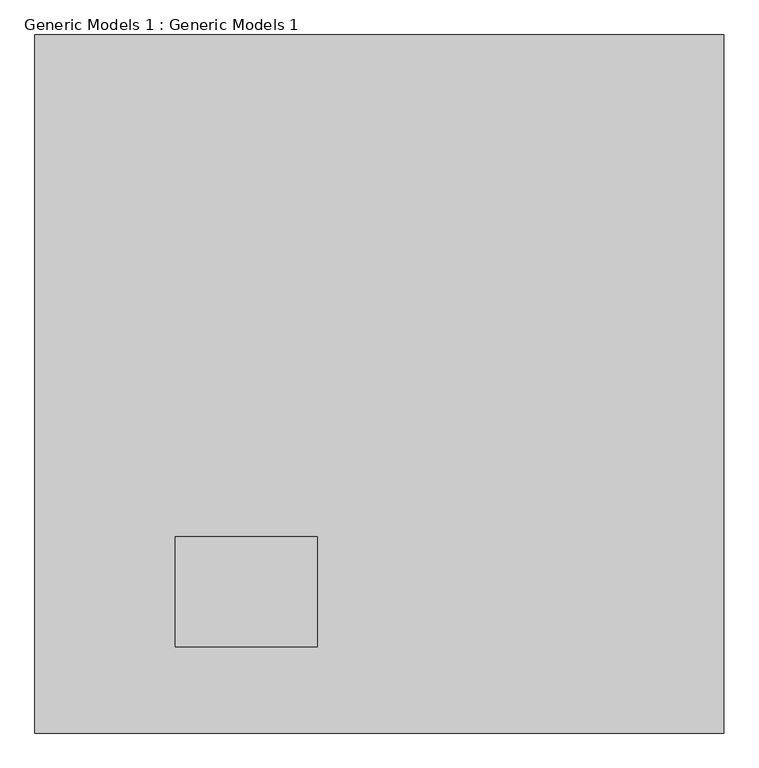
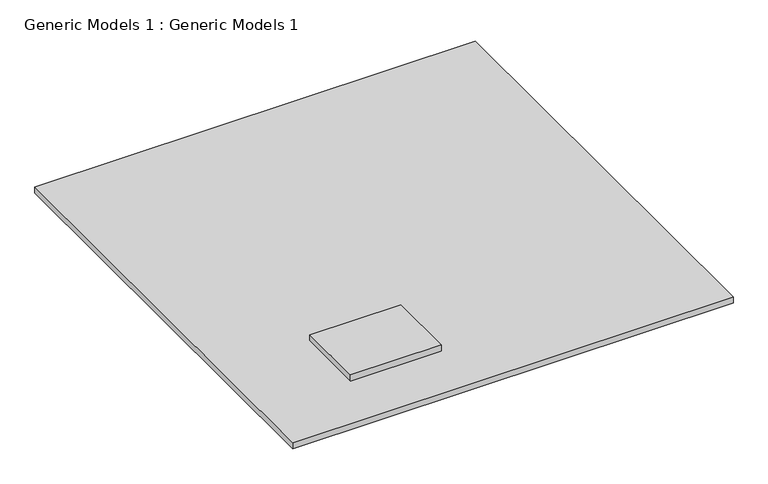
"""IFC4 building model written with IfcOpenShell, lengths in millimetres: proxy geometry, Generic Models 1 : Generic Models 1."""

from ifc_helpers import new_model, si_unit, frame, origin, origin_with_axes, place, context, project, spatial, polyline, outline, extrude, source, transform, mapped, element, save


def generic_models_1_generic_models_1_6e4baba8(model_context):
    return source(origin(), model_context, "Body", "SweptSolid", [
        extrude(outline(polyline([(-2768.0403308, 4700.0157417), (-2768.0403308, -15908.0518738), (-23105.7930973, -15908.0518738), (-23105.7930973, 4700.0157417), (-2768.0403308, 4700.0157417)])), frame((0.0, 0.0, -304.8), z_axis=(0.0, 0.0, 1.0), x_axis=(1.0, 0.0, 0.0)), (0.0, 0.0, 1.0), 304.8),
        extrude(outline(polyline([(-14769.5403308, -10116.8518738), (-14769.5403308, -13355.3518738), (-18960.5403308, -13355.3518738), (-18960.5403308, -10116.8518738), (-14769.5403308, -10116.8518738)])), origin_with_axes(), (0.0, 0.0, 1.0), 304.8),
    ])


if __name__ == "__main__":
    model = new_model("IFC4")
    model_context = context("Model", 3, world=origin())
    ifc_project = project(units=[si_unit("LENGTHUNIT", "METRE", prefix="MILLI")], contexts=[model_context])
    site = spatial("IfcSite", under=ifc_project)
    building = spatial("IfcBuilding", under=site)
    placement = place(None, origin())
    generic_models_1_generic_models_1_shape = generic_models_1_generic_models_1_6e4baba8(model_context)
    element("IfcBuildingElementProxy", 1, Name="Generic Models 1 : Generic Models 1", ObjectType="Generic Models 1 : Generic Models 1", at=placement, inside=building, context=model_context, shape_type="MappedRepresentation", body=[
        mapped(generic_models_1_generic_models_1_shape, transform((0.0, 0.0, 0.0), x_axis=(1.0, 0.0, 0.0), y_axis=(0.0, 1.0, 0.0), z_axis=(0.0, 0.0, 1.0))),
    ])
    save(model, "model.ifc")
